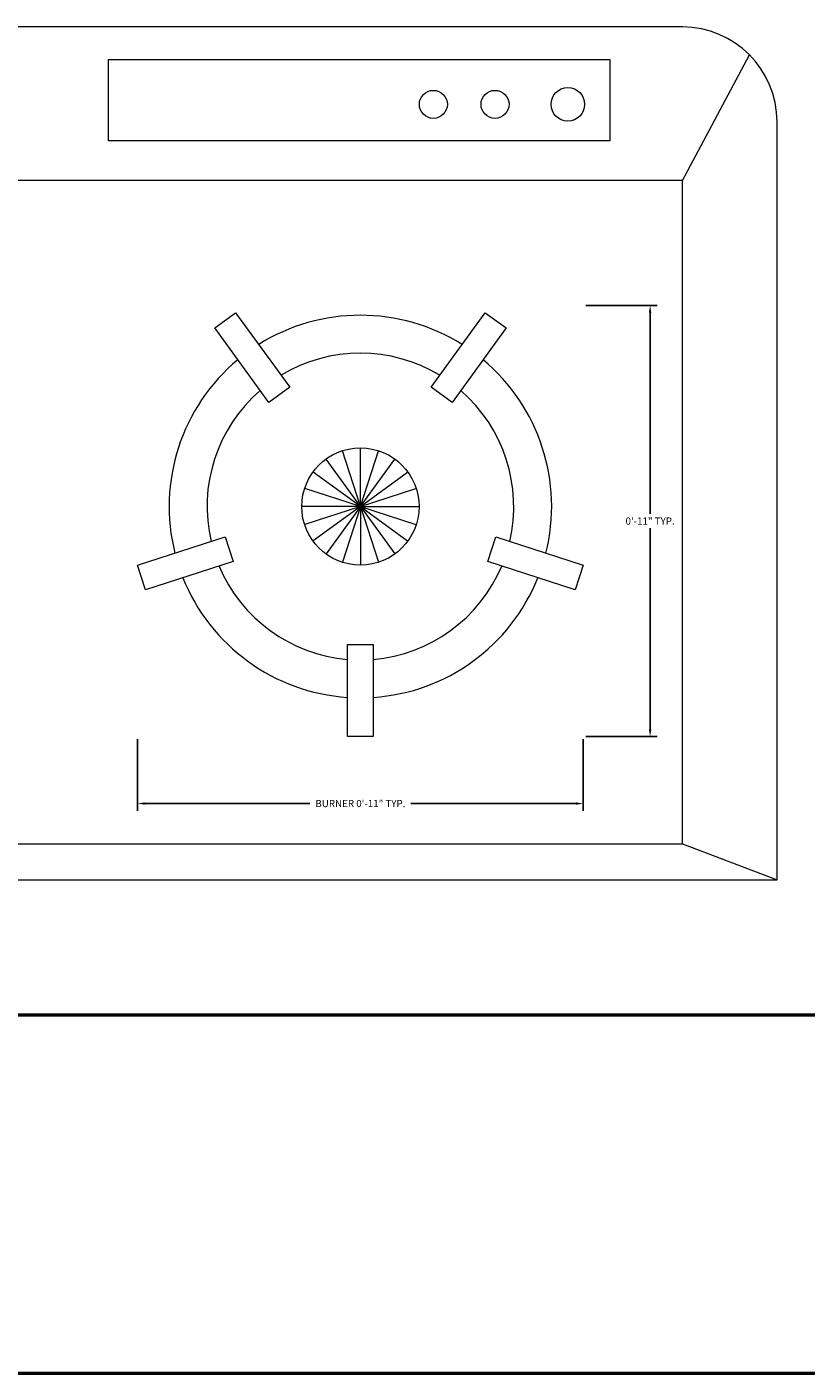
# Model space of a CAD drawing. Units: inches. Extents: x -173 to 545, y -746 to 104.
# Tile 11 of 32: x 320 to 339, y -697 to -664. Entities that reach past the tile are written whole.
import ezdxf

# ---------------------------------------------------------------- set-up
doc = ezdxf.new("R2010")
doc.units = ezdxf.units.IN
doc.header["$MEASUREMENT"] = 0
for name, color, linetype, lineweight in [('A-ANNO-DIMS', 2, 'Continuous', 18), ('A-EQPM', 8, 'Continuous', 18), ('A-WALL', 7, 'Continuous', 50)]:
    doc.layers.add(name, color=color, linetype=linetype, lineweight=lineweight)
doc.styles.get("Standard").update_dxf_attribs({"font": 'arial.ttf'})
doc.dimstyles.get("Standard").update_dxf_attribs({"dimtxt": 0.18, "dimasz": 0.18, "dimexe": 0.18, "dimexo": 0.0625, "dimgap": 0.09, "dimtad": 0, "dimtih": 1, "dimtoh": 1, "dimdec": 0, "dimzin": 0, "dimdsep": 46, "dimlunit": 3, "dimtxsty": 'Standard', "dimcen": 0.09, "dimadec": 0, "dimazin": 0, "dimtfac": 1, "dimtdec": 0, "dimtofl": 0, "dimtmove": 0, "dimatfit": 3, "dimfxl": 1, "dimtolj": 1, "dimtzin": 0, "dimarcsym": 0})

# ---------------------------------------------------------------- blocks, each defined once
blk = doc.blocks.new('HOB-38-BURNER')
for p, q in [((1.939, 10.273), (2.465, 10.656)), ((2.465, 10.656), (3.825, 8.784)), ((7.38, 8.784), (8.739, 10.656)), ((8.739, 10.656), (9.265, 10.273)), ((3.299, 8.402), (1.939, 10.273)), ((9.265, 10.273), (7.906, 8.402)), ((3.825, 8.784), (3.299, 8.402)), ((7.906, 8.402), (7.38, 8.784)), ((5.602, 5.784), (5.149, 7.18)), ((5.602, 5.784), (5.602, 7.251)), ((5.602, 5.784), (6.056, 7.18)), ((5.602, 5.784), (4.74, 6.971)), ((5.602, 5.784), (6.465, 6.971)), ((5.602, 5.784), (4.415, 6.647)), ((5.602, 5.784), (6.789, 6.647)), ((5.602, 5.784), (4.207, 6.238)), ((5.602, 5.784), (6.997, 6.238)), ((5.602, 5.784), (4.135, 5.784)), ((5.602, 5.784), (4.207, 5.331)), ((5.602, 5.784), (4.415, 4.922)), ((5.602, 5.784), (4.74, 4.598)), ((5.602, 5.784), (5.149, 4.389)), ((5.602, 5.784), (7.069, 5.784)), ((5.602, 5.784), (6.997, 5.331)), ((5.602, 5.784), (6.789, 4.922)), ((5.602, 5.784), (6.465, 4.598)), ((5.602, 5.784), (6.056, 4.389)), ((5.602, 5.784), (5.602, 4.317)), ((0, 4.306), (2.2, 5.021)), ((2.2, 5.021), (2.401, 4.402)), ((8.804, 4.402), (9.005, 5.021)), ((9.005, 5.021), (11.204, 4.306)), ((2.401, 4.402), (0.201, 3.688)), ((11.003, 3.688), (8.804, 4.402)), ((0.201, 3.688), (0, 4.306)), ((11.204, 4.306), (11.003, 3.688)), ((5.277, 2.313), (5.927, 2.313)), ((5.277, 0), (5.277, 2.313)), ((5.927, 2.313), (5.927, 0)), ((5.927, 0), (5.277, 0))]:
    blk.add_line(p, q)
blk.add_circle((5.602, 5.784), 1.474)
for radius, start, end in [(4.808, 57.8765, 122.1235), (4.808, 129.8765, 194.1235), (3.855, 58.8365, 121.1635), (4.808, 345.8765, 50.1235), (3.855, 130.8365, 193.1635), (3.855, 346.8365, 49.1635), (3.855, 202.8365, 265.1635), (3.855, 274.8365, 337.1635), (4.808, 201.8765, 266.1235), (4.808, 273.8765, 338.1235)]:
    blk.add_arc((5.602, 5.784), radius, start, end)
blk = doc.blocks.new('*D72')
at = {"layer": 'A-ANNO-DIMS', "color": 0, "lineweight": -2, "transparency": 16777216}
for p, q in [((322.56, -681.43), (322.56, -683.228)), ((333.765, -681.43), (333.765, -683.228)), ((322.74, -683.048), (326.892, -683.048)), ((333.585, -683.048), (329.433, -683.048))]:
    blk.add_line(p, q, dxfattribs=at)
at = {"layer": 'A-ANNO-DIMS', "color": 0, "transparency": 16777216}
for points in [[(322.74, -683.018), (322.74, -683.078), (322.56, -683.048)], [(333.585, -683.018), (333.585, -683.078), (333.765, -683.048)]]:
    blk.add_solid(points, dxfattribs=at)
at = {"layer": 'Defpoints', "color": 0, "transparency": 16777216}
for p in [(322.56, -681.367), (333.765, -681.367), (333.765, -683.048)]:
    blk.add_point(p, dxfattribs=at)
at = {"layer": 'A-ANNO-DIMS', "color": 0, "transparency": 16777216, "insert": (328.162, -683.048), "char_height": 0.18, "attachment_point": 5}
blk.add_mtext('\\A1;BURNER 0\'-11" TYP.', dxfattribs=at)
blk = doc.blocks.new('*D73')
at = {"layer": 'A-ANNO-DIMS', "color": 0, "lineweight": -2, "transparency": 16777216}
for p, q in [((333.827, -670.529), (335.625, -670.529)), ((335.445, -670.709), (335.445, -675.766)), ((335.445, -681.187), (335.445, -676.13)), ((333.827, -681.367), (335.625, -681.367))]:
    blk.add_line(p, q, dxfattribs=at)
at = {"layer": 'A-ANNO-DIMS', "color": 0, "transparency": 16777216}
for points in [[(335.415, -670.709), (335.475, -670.709), (335.445, -670.529)], [(335.415, -681.187), (335.475, -681.187), (335.445, -681.367)]]:
    blk.add_solid(points, dxfattribs=at)
at = {"layer": 'Defpoints', "color": 0, "transparency": 16777216}
for p in [(333.765, -670.529), (335.445, -670.529), (333.765, -681.367)]:
    blk.add_point(p, dxfattribs=at)
at = {"layer": 'A-ANNO-DIMS', "color": 0, "transparency": 16777216, "insert": (335.445, -675.948), "char_height": 0.18, "attachment_point": 5}
blk.add_mtext('\\A1;0\'-11" TYP.', dxfattribs=at)

msp = doc.modelspace()

# ---------------------------------------------------------------- linework, layer by layer
at = {"layer": 'A-EQPM'}
for p, q in [((336.255, -663.529), (302.912, -663.529)), ((321.826, -664.349), (334.434, -664.349)), ((321.826, -666.39), (321.826, -664.349)), ((334.434, -664.349), (334.434, -666.39)), ((336.255, -667.388), (337.939, -664.227)), ((338.637, -684.964), (338.637, -665.911)), ((334.434, -666.39), (321.826, -666.39)), ((336.255, -667.388), (302.912, -667.388)), ((336.255, -684.059), (336.255, -667.388)), ((302.912, -684.059), (336.255, -684.059)), ((336.255, -684.059), (338.637, -684.964)), ((300.53, -684.964), (338.637, -684.964))]:
    msp.add_line(p, q, dxfattribs=at)
for centre, radius in [((329.996, -665.475), 0.352), ((331.546, -665.475), 0.352), ((333.377, -665.475), 0.422)]:
    msp.add_circle(centre, radius, dxfattribs=at)
msp.add_arc((336.255, -665.911), 2.382, 0, 90, dxfattribs=at)
at = {"layer": 'A-WALL'}
for p, q in [((265.301, -688.362), (356.301, -688.362)), ((24.301, -697.362), (501.801, -697.362))]:
    msp.add_line(p, q, dxfattribs=at)

# ---------------------------------------------------------------- block references
at = {"layer": 'A-EQPM'}
msp.add_blockref('HOB-38-BURNER', (322.56, -681.367), dxfattribs=at)

# ---------------------------------------------------------------- dimensions: what is measured, and where the dimension line sits
at = {"layer": 'A-ANNO-DIMS'}
dim = msp.add_linear_dim(base=(335.445, -670.529), p1=(333.765, -681.367), p2=(333.765, -670.529), angle=90, text='<> TYP.', dimstyle='Standard', override={"dimdec": 1, "dimlfac": 1, "dimrnd": 0, "dimzin": 1, "dimdsep": 46, "dimlunit": 4, "dimfrac": 2}, dxfattribs=at)
dim.commit()
dim.dimension.update_dxf_attribs({"geometry": '*D73', "text_midpoint": (335.445, -675.948)})
dim = msp.add_linear_dim(base=(333.765, -683.048), p1=(322.56, -681.367), p2=(333.765, -681.367), text='BURNER <> TYP.', dimstyle='Standard', override={"dimdec": 1, "dimlfac": 1, "dimrnd": 0, "dimzin": 1, "dimdsep": 46, "dimlunit": 4, "dimfrac": 2}, dxfattribs=at)
dim.commit()
dim.dimension.update_dxf_attribs({"geometry": '*D72', "text_midpoint": (328.162, -683.048)})

doc.saveas('drawing.dxf')
